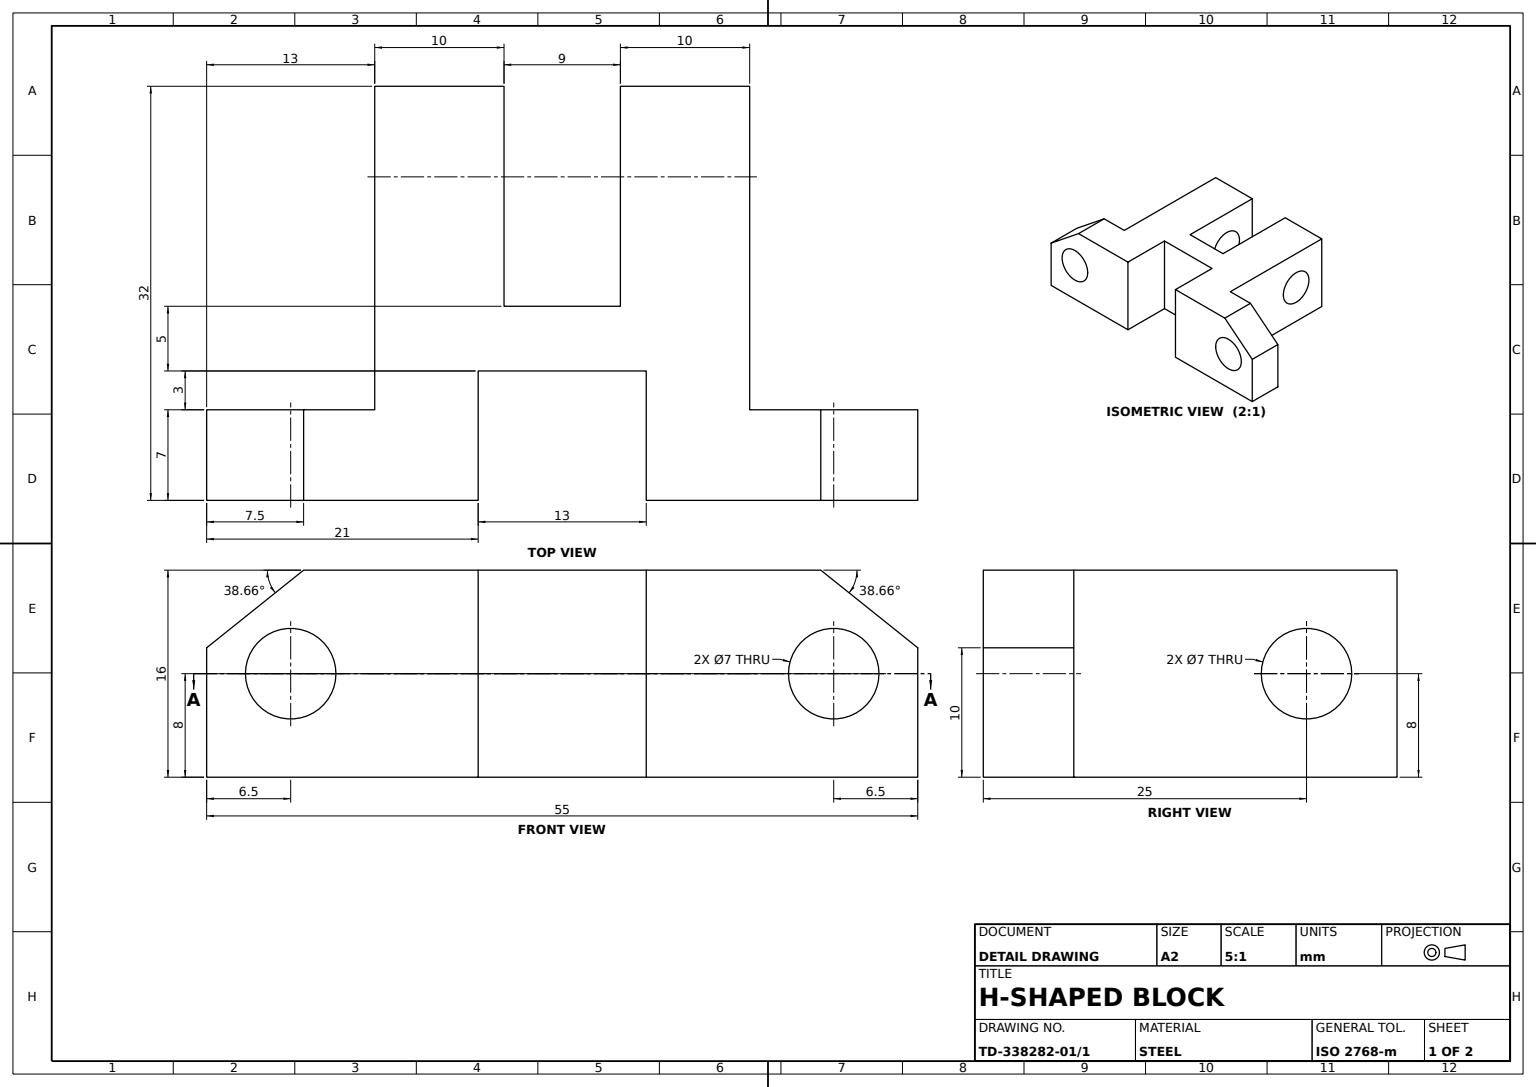
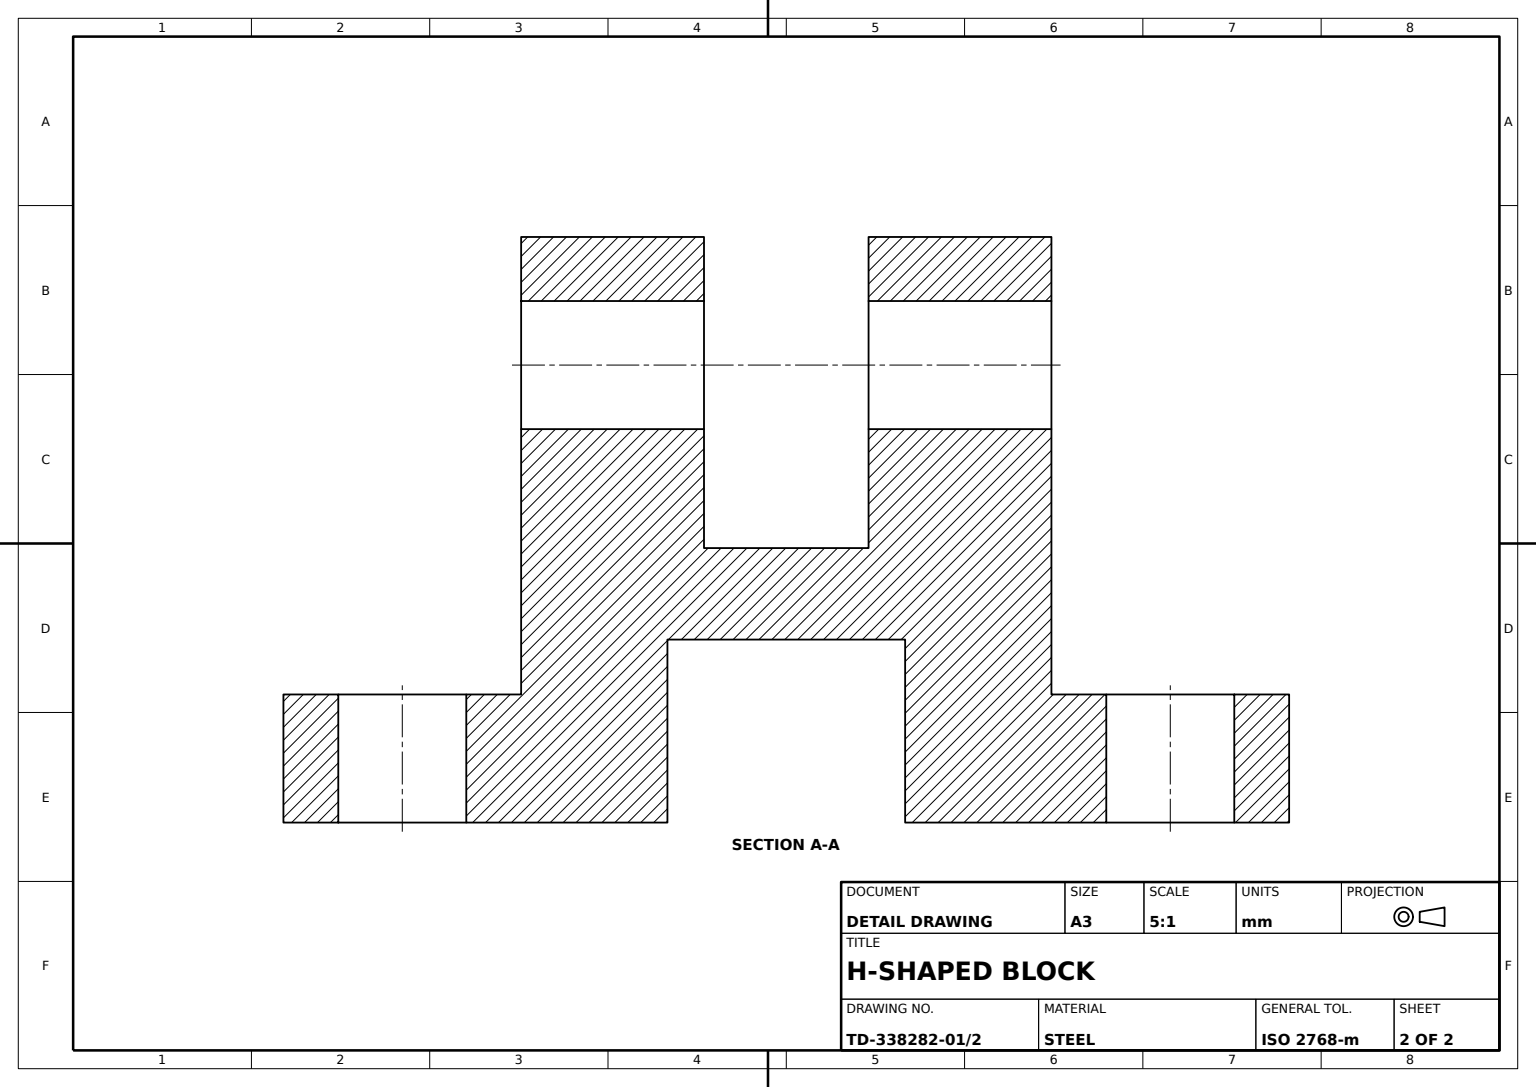
from build123d import *

# Parameters (mm, degrees)
BASE_BLOCK_PROFILE_W        = 55
BASE_BLOCK_PROFILE_H        = 16
BASE_BLOCK_DEPTH            = 32
CENTRE_NOTCH_DEPTH          = 46.124826869
CENTRE_NOTCH_DEPTH_BACK     = 46.124826869
CENTRE_NOTCH_PROFILE_W      = 13
CENTRE_NOTCH_PROFILE_H      = 25
SIDE_STEP_CUT_DEPTH         = 46.124826869
SIDE_STEP_CUT_DEPTH_BACK    = 46.124826869
SIDE_STEP_CUT_PROFILE_W     = 13
SIDE_STEP_CUT_PROFILE_H     = 10
CORNER_BEVEL_CUT_DEPTH      = 46.124826869
CORNER_BEVEL_CUT_DEPTH_BACK = 46.124826869
CORNER_BEVEL_PROFILE_W      = 9
CORNER_BEVEL_PROFILE_H      = 17
LUG_SLOT_CUT_DEPTH          = 39.016443811
LUG_SLOT_CUT_DEPTH_BACK     = 39.016443811
LUG_HOLES_7_DEPTH           = 39.016443811
LUG_HOLES_7_DEPTH_BACK      = 39.016443811
LUG_HOLES_7_SKETCH_R        = 3.5
CROSS_HOLE_7_DEPTH          = 54.404119691
CROSS_HOLE_7_DEPTH_BACK     = 54.404119691
CROSS_HOLE_7_SKETCH_R       = 3.5


with BuildPart() as part:
    # Base Block Profile → Base Block (new body)
    with BuildSketch(Plane.XY):
        Rectangle(BASE_BLOCK_PROFILE_W, BASE_BLOCK_PROFILE_H)
    extrude(amount=BASE_BLOCK_DEPTH)

    # Centre Notch Profile → Centre Notch (cut, two sides: drawn at the far end of the back side and taken through both)
    with BuildSketch(Plane(origin=(0, 8, 0), x_dir=(1, 0, 0), z_dir=(0, 1, 0)).offset(-CENTRE_NOTCH_DEPTH_BACK)):
        with Locations((-21, -12.5)):
            Rectangle(CENTRE_NOTCH_PROFILE_W, CENTRE_NOTCH_PROFILE_H)
        with Locations((21, -12.5)):
            Rectangle(CENTRE_NOTCH_PROFILE_W, CENTRE_NOTCH_PROFILE_H)
    extrude(amount=CENTRE_NOTCH_DEPTH + CENTRE_NOTCH_DEPTH_BACK, mode=Mode.SUBTRACT)

    # Side Step Cut Profile → Side Step Cut (cut, two sides: drawn at the far end of the back side and taken through both)
    with BuildSketch(Plane(origin=(0, 8, 0), x_dir=(1, 0, 0), z_dir=(0, 1, 0)).offset(-SIDE_STEP_CUT_DEPTH_BACK)):
        with Locations((0, -27)):
            Rectangle(SIDE_STEP_CUT_PROFILE_W, SIDE_STEP_CUT_PROFILE_H)
    extrude(amount=SIDE_STEP_CUT_DEPTH + SIDE_STEP_CUT_DEPTH_BACK, mode=Mode.SUBTRACT)

    # Corner Bevel Profile → Corner Bevel Cut (cut, two sides: drawn at the far end of the back side and taken through both)
    with BuildSketch(Plane(origin=(0, 8, 0), x_dir=(1, 0, 0), z_dir=(0, 1, 0)).offset(-CORNER_BEVEL_CUT_DEPTH_BACK)):
        with Locations((0, -8.5)):
            Rectangle(CORNER_BEVEL_PROFILE_W, CORNER_BEVEL_PROFILE_H)
    extrude(amount=CORNER_BEVEL_CUT_DEPTH + CORNER_BEVEL_CUT_DEPTH_BACK, mode=Mode.SUBTRACT)

    # Lug Slot Profile → Lug Slot Cut (cut, two sides: drawn at the far end of the back side and taken through both)
    with BuildSketch(Plane(origin=(0, 0, 25), x_dir=(-1, 0, 0), z_dir=(0, 0, -1)).offset(-LUG_SLOT_CUT_DEPTH_BACK)):
        Polygon((-27.5, 8), (-20, 8), (-27.5, 2), align=None)
        Polygon((20, 8), (27.5, 2), (27.5, 8), align=None)
    extrude(amount=LUG_SLOT_CUT_DEPTH + LUG_SLOT_CUT_DEPTH_BACK, mode=Mode.SUBTRACT)

    # Lug Holes Ø7 Sketch → Lug Holes Ø7 (cut, two sides: drawn at the far end of the back side and taken through both)
    with BuildSketch(Plane(origin=(0, 0, 25), x_dir=(-1, 0, 0), z_dir=(0, 0, -1)).offset(-LUG_HOLES_7_DEPTH_BACK)):
        with BuildLine():
            ThreePointArc((24.5, 0), (21, 3.5), (17.5, 0))
            Line((17.5, 0), (24.5, 0))
        make_face()
        with BuildLine():
            Line((24.5, 0), (17.5, 0))
            ThreePointArc((17.5, 0), (21, -3.5), (24.5, 0))
        make_face()
        with Locations((-21, 0)):
            Circle(LUG_HOLES_7_SKETCH_R)
    extrude(amount=LUG_HOLES_7_DEPTH + LUG_HOLES_7_DEPTH_BACK, mode=Mode.SUBTRACT)

    # Cross Hole Ø7 Sketch → Cross Hole Ø7 (cut, two sides: drawn at the far end of the back side and taken through both)
    with BuildSketch(Plane(origin=(14.5, 0, 0), x_dir=(0, 0, -1), z_dir=(1, 0, 0)).offset(-CROSS_HOLE_7_DEPTH_BACK)):
        with Locations((-7, 0)):
            Circle(CROSS_HOLE_7_SKETCH_R)
    extrude(amount=CROSS_HOLE_7_DEPTH + CROSS_HOLE_7_DEPTH_BACK, mode=Mode.SUBTRACT)


solid = part.part
